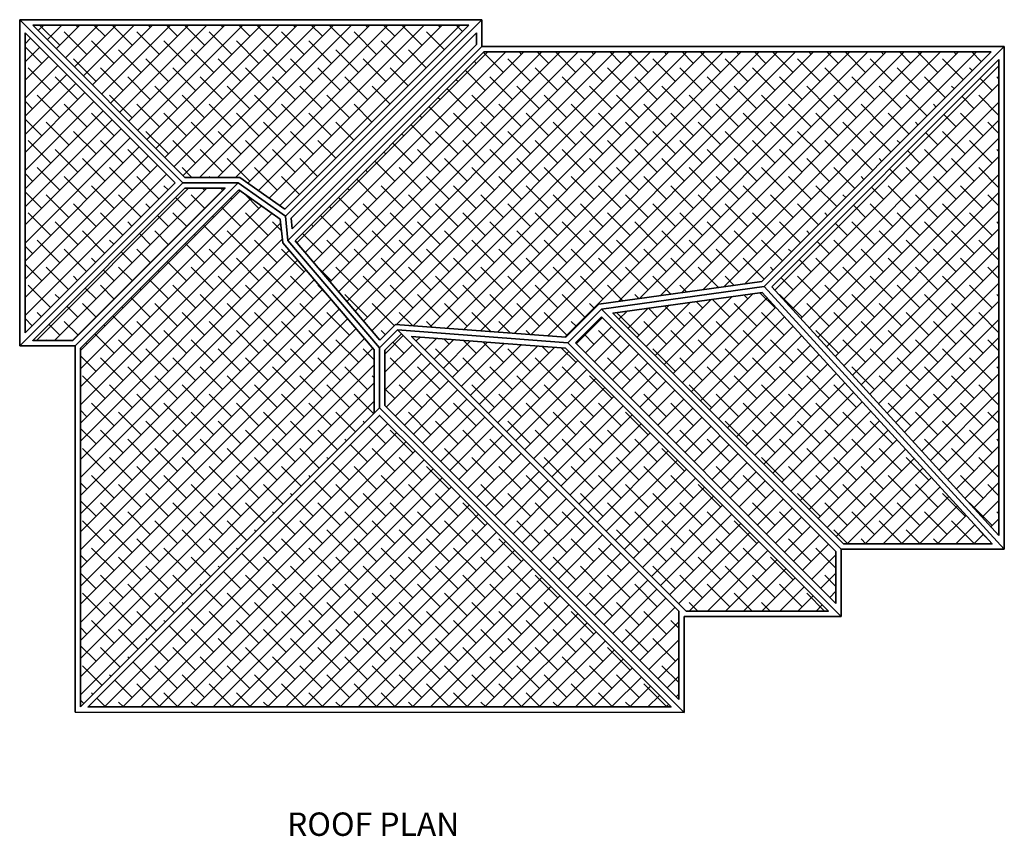
# Model space of a CAD drawing. Units: millimetres. Extents: x -857 to 54106, y -13666 to 13947.
# Tile 41 of 41: x 39456 to 54106, y 1561 to 13704. Entities that reach past the tile are written whole.
import ezdxf

# ---------------------------------------------------------------- set-up
doc = ezdxf.new("R2010")
doc.units = ezdxf.units.MM
for name, color, linetype, lineweight in [('A-ANNO-TEXT', 7, 'Continuous', 25), ('A-ROOF', 7, 'Continuous', 35), ('A-ROOF-PATT', 252, 'Continuous', 13)]:
    doc.layers.add(name, color=color, linetype=linetype, lineweight=lineweight)
doc.styles.get("Standard").update_dxf_attribs({"font": 'arial.ttf'})

msp = doc.modelspace()

# ---------------------------------------------------------------- hatches: boundary and pattern name
at = {"layer": 'A-ROOF-PATT'}
h = msp.add_hatch(dxfattribs=at)
h.set_pattern_fill('ANSI38', color=256, scale=60)
h.set_pattern_definition([(45, (-22719.68, -12808.97), (-134.70384, 134.70384), []), (135, (-22719.68, -12808.97), (-404.11153, 134.70384), [476.25, -285.75])])
h.paths.add_polyline_path([(44730.453, 7853.948), (44730.453, 8793.637), (43368.626, 10386.301), (43333.673, 10738.804), (42714.743, 11175.046), (40360.791, 8821.094), (40360.791, 3484.286)])
h.paths.add_polyline_path([(45441.766, 7189.499), (44810.453, 7820.811), (40473.917, 3484.275), (49147.483, 3483.782)])
h.paths.add_polyline_path([(45934.996, 8234.865), (45135.138, 9034.724), (44890.453, 8790.039), (44890.453, 7967.085), (45554.903, 7302.636), (49260.631, 3596.908), (49260.631, 4909.231)])
h.paths.add_polyline_path([(47575.77, 8821.115), (45287.857, 8995.142), (45991.565, 8291.434), (49373.768, 4909.231), (51487.654, 4909.231)])
h.paths.add_polyline_path([(48111.385, 9285.5), (47724.522, 8898.637), (51600.791, 5022.368), (51600.791, 5796.094)])
h.paths.add_polyline_path([(50503.671, 9649.512), (48281.679, 9341.48), (51713.928, 5909.231), (53924.227, 5909.231)])
h.paths.add_polyline_path([(50496.761, 9810.085), (53912.593, 13224.231), (46363.928, 13224.231), (43554.646, 10414.949), (44815.045, 8940.905), (45047.99, 9173.849), (47580.805, 8981.194), (48073.803, 9474.192)])
h.paths.add_polyline_path([(54025.798, 13111.161), (50645.012, 9732.045), (54025.798, 6035.251)])
h.paths.add_polyline_path([(46137.654, 13624.231), (39648.928, 13624.231), (41913.928, 11359.231), (42731.151, 11359.231), (43400.72, 10887.297)])
h.paths.add_polyline_path([(39535.791, 13511.094), (39535.791, 9047.368), (41767.654, 11279.231)])
h.paths.add_polyline_path([(42512.654, 11199.231), (41913.928, 11199.231), (39648.928, 8934.231), (40247.654, 8934.231)])

# ---------------------------------------------------------------- linework, layer by layer
at = {"layer": 'A-ROOF'}
for p, q in [((39455.791, 13704.231), (41880.791, 11279.231)), ((39455.791, 13704.231), (46330.791, 13704.231)), ((39455.791, 8854.231), (39455.791, 13704.231)), ((46330.791, 13704.231), (43409.672, 10783.112)), ((46330.791, 13704.231), (46330.791, 13304.231)), ((39535.791, 9047.368), (39535.791, 13511.094)), ((39535.791, 13511.094), (41767.654, 11279.231)), ((39648.928, 13624.231), (46137.654, 13624.231)), ((39648.928, 13624.231), (41913.928, 11359.231)), ((46137.654, 13624.231), (43400.72, 10887.297)), ((46137.654, 13624.231), (43400.72, 10887.297)), ((46250.791, 13511.094), (43493.019, 10753.322)), ((46250.791, 13511.094), (46250.791, 13337.368)), ((46250.791, 13337.368), (43508.69, 10595.267)), ((46330.791, 13304.231), (43445.756, 10419.196)), ((46363.928, 13224.231), (43554.646, 10414.949)), ((46330.791, 13304.231), (54105.798, 13304.231)), ((46363.928, 13224.231), (53912.593, 13224.231)), ((53912.593, 13224.231), (50496.761, 9810.085)), ((54105.798, 13304.231), (50534.332, 9734.528)), ((54105.798, 13304.231), (54105.798, 5829.231)), ((54025.798, 13111.161), (50645.012, 9732.045)), ((54025.798, 13111.161), (54025.798, 6035.251)), ((41913.928, 11359.231), (42731.151, 11359.231)), ((42731.151, 11359.231), (43400.72, 10887.297)), ((39455.791, 8854.231), (41880.791, 11279.231)), ((39535.791, 9047.368), (41767.654, 11279.231)), ((40280.791, 8854.231), (42705.791, 11279.231)), ((40360.791, 8821.094), (42714.743, 11175.046)), ((41880.791, 11279.231), (42705.791, 11279.231)), ((42705.791, 11279.231), (43409.672, 10783.112)), ((42705.791, 11279.231), (43409.672, 10783.112)), ((42714.743, 11175.046), (43333.673, 10738.804)), ((43333.673, 10738.804), (43368.626, 10386.301)), ((43409.672, 10783.112), (43445.756, 10419.196)), ((43493.019, 10753.322), (43508.69, 10595.267)), ((43445.756, 10419.196), (44810.453, 8823.176)), ((43554.646, 10414.949), (44815.045, 8940.905)), ((43368.626, 10386.301), (44730.453, 8793.637)), ((48073.803, 9474.192), (50496.761, 9810.085)), ((48111.385, 9398.637), (50534.332, 9734.528)), ((54105.798, 5829.231), (50534.332, 9734.528)), ((54025.798, 6035.251), (50645.012, 9732.045)), ((48073.803, 9474.192), (47580.805, 8981.194)), ((48111.385, 9398.637), (47611.385, 8898.637)), ((51680.791, 5829.231), (48111.385, 9398.637)), ((48111.385, 9285.5), (47724.522, 8898.637)), ((51600.791, 5796.094), (48111.385, 9285.5)), ((44810.453, 8823.176), (45078.57, 9091.292)), ((44815.045, 8940.905), (45047.99, 9173.849)), ((44815.045, 8940.905), (45022.001, 9147.861)), ((47580.805, 8981.194), (45047.99, 9173.849)), ((45934.996, 8234.865), (45078.57, 9091.292)), ((47611.385, 8898.637), (45078.57, 9091.292)), ((44890.453, 8790.039), (45135.138, 9034.724)), ((40280.791, 8854.231), (39455.791, 8854.231)), ((40280.791, 3404.286), (40280.791, 8854.231)), ((40360.791, 3484.286), (40360.791, 8821.094)), ((44730.453, 7853.948), (44730.453, 8793.637)), ((44753.885, 8879.744), (44758.304, 8884.164)), ((44810.453, 7933.948), (44810.453, 8823.176)), ((44890.453, 7967.085), (44890.453, 8790.039)), ((51680.791, 4829.231), (47611.385, 8898.637)), ((51600.791, 5022.368), (47724.522, 8898.637)), ((49260.631, 4909.231), (45934.996, 8234.865)), ((40360.791, 3484.286), (44810.453, 7933.948)), ((45498.334, 7246.067), (44810.453, 7933.948)), ((45554.903, 7302.636), (44890.453, 7967.085)), ((49340.631, 3403.771), (45498.334, 7246.067)), ((49260.631, 3596.908), (45554.903, 7302.636)), ((51600.791, 5796.094), (51600.791, 5022.368)), ((54105.798, 5829.231), (51680.791, 5829.231)), ((51680.791, 5829.231), (51680.791, 4829.231)), ((49260.631, 4909.231), (49260.631, 3596.908)), ((51680.791, 4829.231), (49340.631, 4829.231)), ((49340.631, 4829.231), (49340.631, 3403.771)), ((49340.631, 3403.771), (40280.791, 3404.286))]:
    msp.add_line(p, q, dxfattribs=at)
for points in [[(41913.928, 11199.231), (39648.928, 8934.231), (40247.654, 8934.231), (42512.654, 11199.231)], [(50503.671, 9649.512), (53924.227, 5909.231), (51713.928, 5909.231), (48281.679, 9341.48)], [(47575.77, 8821.115), (51487.654, 4909.231), (49373.768, 4909.231), (45991.565, 8291.434), (45287.857, 8995.142)], [(45441.766, 7189.499), (49147.483, 3483.782), (40473.917, 3484.275), (44810.453, 7820.811)]]:
    msp.add_lwpolyline(points, close=True, dxfattribs=at)

# ---------------------------------------------------------------- texts
at = {"layer": 'A-ANNO-TEXT', "insert": (43434.156, 1914.444), "char_height": 347.60543, "attachment_point": 1}
msp.add_mtext_dynamic_manual_height_columns('\\pxt0;ROOF PLAN', width=5900.0263, gutter_width=43450.679, heights=[5996.136], dxfattribs=at)

doc.saveas('drawing.dxf')
